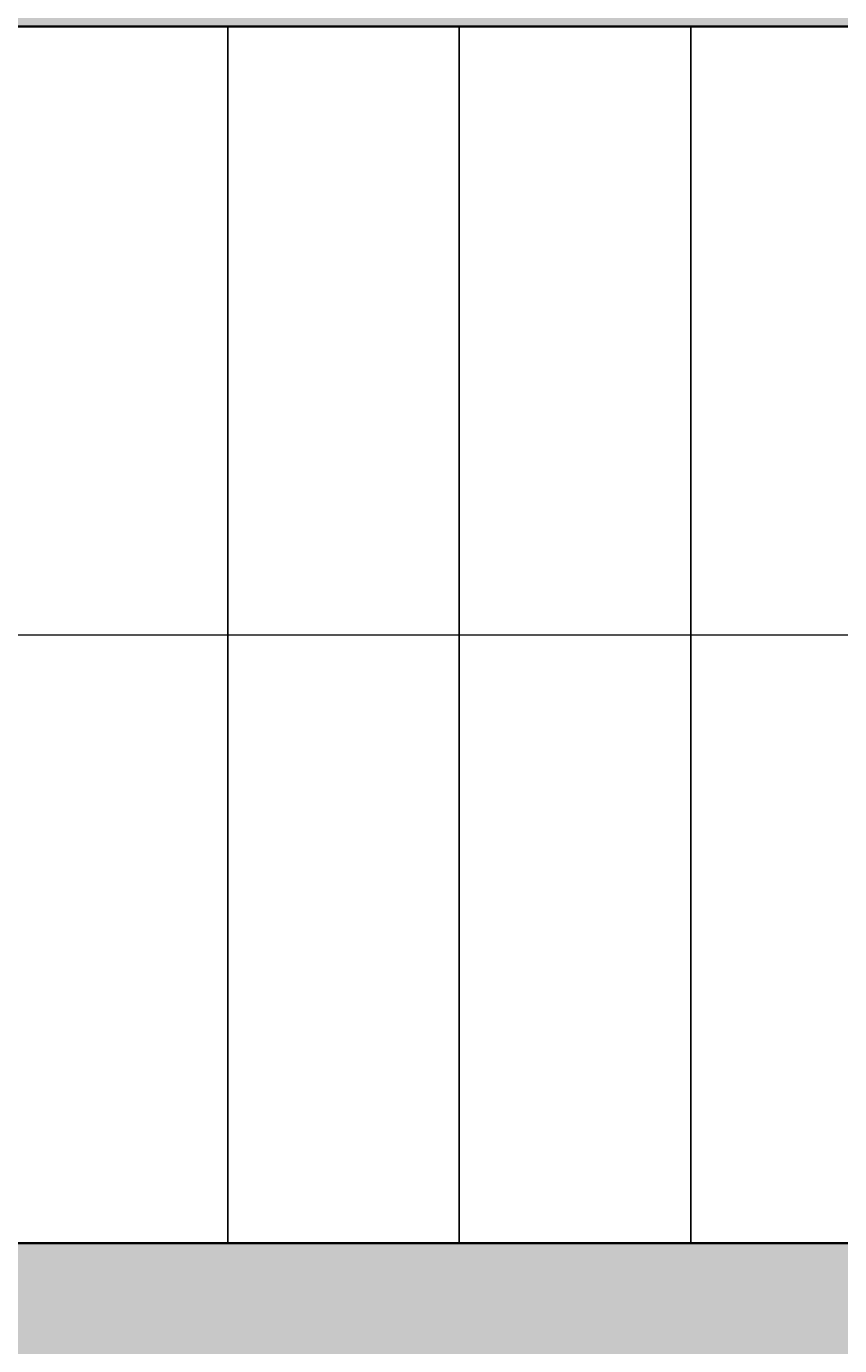
# Model space of a CAD drawing. Units: inches. Extents: x 1998 to 2588, y 1139 to 1977.
# Tile 89 of 134: x 2425 to 2453, y 1477 to 1523. Entities that reach past the tile are written whole.
import ezdxf

# ---------------------------------------------------------------- set-up
doc = ezdxf.new("R2010")
doc.units = ezdxf.units.IN
for name, color, linetype, lineweight in [('A-ANNO-DIMS', 2, 'Continuous', 18), ('A-ANNO-SYMB', 7, 'Continuous', 18), ('A-FLOR-EVTR', 7, 'Continuous', 35), ('A-FLOR-STRS', 7, 'Continuous', 25), ('A-WALL-PATT', 252, 'Continuous', 13), ('WALL', 200, 'Continuous', 35)]:
    doc.layers.add(name, color=color, linetype=linetype, lineweight=lineweight)
doc.styles.get("Standard").update_dxf_attribs({"font": 'arial.ttf'})
doc.dimstyles.get("Standard").update_dxf_attribs({"dimtxt": 0.18, "dimasz": 0.18, "dimexe": 0.18, "dimexo": 0.0625, "dimgap": 0.09, "dimtad": 0, "dimtih": 1, "dimtoh": 1, "dimdec": 4, "dimzin": 0, "dimdsep": 46, "dimtxsty": 'Standard', "dimcen": 0.09, "dimadec": 0, "dimazin": 0, "dimtfac": 1, "dimtdec": 4, "dimtofl": 0, "dimtmove": 0, "dimatfit": 3, "dimfxl": 1, "dimtolj": 1, "dimtzin": 0, "dimarcsym": 0})

# ---------------------------------------------------------------- blocks, each defined once
blk = doc.blocks.new('*D24')
at = {"layer": 'A-ANNO-DIMS', "color": 0, "lineweight": -2, "transparency": 16777216}
for p, q in [((2398.535, 1911.232), (2588.309, 1911.232)), ((2588.129, 1911.052), (2588.129, 1570.164)), ((2588.129, 1228.912), (2588.129, 1569.8)), ((2527.535, 1228.732), (2588.309, 1228.732))]:
    blk.add_line(p, q, dxfattribs=at)
at = {"layer": 'A-ANNO-DIMS', "color": 0, "transparency": 16777216}
for points in [[(2588.099, 1911.052), (2588.159, 1911.052), (2588.129, 1911.232)], [(2588.099, 1228.912), (2588.159, 1228.912), (2588.129, 1228.732)]]:
    blk.add_solid(points, dxfattribs=at)
at = {"layer": 'Defpoints', "color": 0, "transparency": 16777216}
for p in [(2398.473, 1911.232), (2588.129, 1911.232), (2527.473, 1228.732)]:
    blk.add_point(p, dxfattribs=at)
at = {"layer": 'A-ANNO-DIMS', "color": 0, "transparency": 16777216, "insert": (2588.129, 1569.982), "char_height": 0.18, "attachment_point": 5}
blk.add_mtext('\\A1;682.5', dxfattribs=at)
blk = doc.blocks.new('*D33')
at = {"layer": 'A-ANNO-DIMS', "color": 0, "lineweight": -2, "transparency": 16777216}
for p, q in [((2407.973, 1480.67), (2407.973, 1138.602)), ((2498.179, 1480.67), (2498.179, 1138.602)), ((2408.153, 1138.782), (2452.753, 1138.782)), ((2497.999, 1138.782), (2453.399, 1138.782))]:
    blk.add_line(p, q, dxfattribs=at)
at = {"layer": 'A-ANNO-DIMS', "color": 0, "transparency": 16777216}
for points in [[(2408.153, 1138.812), (2408.153, 1138.752), (2407.973, 1138.782)], [(2497.999, 1138.812), (2497.999, 1138.752), (2498.179, 1138.782)]]:
    blk.add_solid(points, dxfattribs=at)
at = {"layer": 'Defpoints', "color": 0, "transparency": 16777216}
for p in [(2407.973, 1480.732), (2498.179, 1480.732), (2498.179, 1138.782)]:
    blk.add_point(p, dxfattribs=at)
at = {"layer": 'A-ANNO-DIMS', "color": 0, "transparency": 16777216, "insert": (2453.076, 1138.782), "char_height": 0.18, "attachment_point": 5}
blk.add_mtext('\\A1;90.2', dxfattribs=at)

msp = doc.modelspace()

# ---------------------------------------------------------------- hatches: boundary and pattern name
at = {"layer": 'A-WALL-PATT'}
h = msp.add_hatch(color=256, dxfattribs=at)
h.dxf.hatch_style = 1
h.paths.add_polyline_path([(2527.4729, 1362.2324), (2510.9729, 1362.2324), (2510.9729, 1357.7324), (2518.4729, 1357.7324), (2518.4729, 1237.7324), (2503.1458, 1237.7324), (2503.1458, 1228.7324), (2527.4729, 1228.7324)])
h.paths.add_polyline_path([(2490.5682, 1362.2324), (2398.4729, 1362.2324), (2398.4729, 1357.7324), (2490.5682, 1357.7324)])
h.paths.add_polyline_path([(2224.9729, 1264.7324), (2222.9729, 1264.7324), (2222.9729, 1232.4125), (2341.4729, 1232.4125), (2341.4729, 1234.4125), (2224.9729, 1234.4125)])
h.paths.add_polyline_path([(2334.5332, 1273.7324), (2264.7638, 1273.7324), (2264.7638, 1269.5611, -0.043659), (2264.3413, 1264.7324), (2334.5332, 1264.7324)])
h.paths.add_polyline_path([(2236.9551, 1273.7324), (2234.4125, 1273.7324), (2234.4125, 1264.7324), (2236.9551, 1264.7324), (2236.9551, 1269.5611)])
h.paths.add_polyline_path([(2222.9729, 1293.2324), (2096.9729, 1293.2324), (2096.9729, 1345.0966), (2087.9729, 1345.0966), (2087.9729, 1284.2324), (2222.9729, 1284.2324), (2222.9729, 1285.137)])
h.paths.add_polyline_path([(2096.9729, 1458.7927), (2087.9729, 1458.7927), (2087.9729, 1417.7324), (2087.9729, 1413.2324), (2096.9729, 1413.2324), (2096.9729, 1417.7324)])
h.paths.add_polyline_path([(2096.9729, 1413.2324), (2087.9729, 1413.2324), (2087.9729, 1365.5012), (2096.9729, 1365.5012), (2096.9729, 1369.3358)])
h.paths.add_polyline_path([(2186.2943, 1417.7324), (2138.6074, 1417.7324), (2096.9729, 1417.7324), (2096.9729, 1413.2324), (2138.6074, 1413.2324), (2186.2943, 1413.2324)])
h.paths.add_polyline_path([(2181.4729, 1465.7324), (2176.9729, 1465.7324), (2176.9729, 1451.6434), (2181.4729, 1451.6434)])
h.paths.add_polyline_path([(2181.4729, 1422.1664), (2176.9729, 1422.1664), (2176.9729, 1417.7324), (2181.4729, 1417.7324)])
h.paths.add_polyline_path([(2063.9729, 1465.7324), (2087.9729, 1465.7324), (2087.9729, 1470.2324), (2059.4729, 1470.2324), (2059.4729, 1413.2324), (2087.9729, 1413.2324), (2087.9729, 1417.7324), (2063.9729, 1417.7324)])
h.paths.add_polyline_path([(2181.4729, 1755.2324), (2176.9729, 1755.2324), (2176.9729, 1748.6798), (2177.0513, 1748.6798), (2181.4729, 1748.6798)])
h.paths.add_polyline_path([(2227.4729, 1707.2324), (2220.4647, 1707.2324), (2220.4647, 1702.7324), (2222.9729, 1702.7324), (2222.9729, 1604.637), (2227.4729, 1604.637)])
h.paths.add_polyline_path([(2114.9729, 1702.7324), (2105.9729, 1702.7324), (2105.9729, 1628.4781, -0.0318759), (2110.1012, 1628.7416), (2114.9729, 1628.7416)])
h.paths.add_polyline_path([(2345.9729, 1739.3278), (2341.4729, 1739.3278), (2341.4729, 1647.5211), (2345.9729, 1647.5211)])
h.paths.add_polyline_path([(2350.6273, 1641.2324), (2345.9729, 1641.2324), (2345.9729, 1636.7324), (2350.6273, 1636.7324), (2350.6273, 1639.8729)])
h.paths.add_polyline_path([(2501.9729, 1641.2324), (2407.9729, 1641.2324), (2392.5005, 1641.2324), (2392.5005, 1639.8729), (2392.5005, 1636.7324), (2501.9729, 1636.7324)])
h.paths.add_polyline_path([(2510.9729, 1755.2324), (2501.9729, 1755.2324), (2501.9729, 1641.2324), (2510.9729, 1641.2324)])
h.paths.add_polyline_path([(2549.1786, 1641.2324), (2522.3775, 1641.2324), (2522.3775, 1636.7324), (2540.1786, 1636.7324), (2540.1786, 1480.7324), (2522.3775, 1480.7324), (2522.3775, 1476.2324), (2549.1786, 1476.2324)])
h.paths.add_polyline_path([(2498.1786, 1594.7324), (2407.9729, 1594.7324), (2407.9729, 1585.7324), (2416.9729, 1585.7324), (2489.1786, 1585.7324), (2489.1786, 1531.7324), (2416.9729, 1531.7324), (2407.9729, 1531.7324), (2407.9729, 1522.7324), (2498.1786, 1522.7324)])
h.paths.add_polyline_path([(2351.6437, 1480.7324), (2345.9729, 1480.7324), (2345.9729, 1476.2324), (2351.6437, 1476.2324), (2351.6437, 1477.5919)])
h.paths.add_polyline_path([(2501.9729, 1480.7324), (2498.1786, 1480.7324), (2407.9729, 1480.7324), (2393.5168, 1480.7324), (2393.5168, 1477.5919), (2393.5168, 1476.2324), (2501.9729, 1476.2324)])

# ---------------------------------------------------------------- linework, layer by layer
at = {"layer": 'A-ANNO-SYMB'}
msp.add_line((2407.9729, 1501.7324), (2498.1786, 1501.7324), dxfattribs=at)
at = {"layer": 'A-FLOR-EVTR'}
msp.add_lwpolyline([(2407.9729, 1522.7324), (2498.1786, 1522.7324), (2498.1786, 1594.7324), (2407.9729, 1594.7324)], close=True, dxfattribs=at)
at = {"layer": 'A-FLOR-STRS'}
for p, q in [((2540.1786, 1522.7324), (2407.9729, 1522.7324)), ((2431.9729, 1480.7324), (2431.9729, 1522.7324)), ((2439.9729, 1480.7324), (2439.9729, 1522.7324)), ((2447.9729, 1480.7324), (2447.9729, 1522.7324))]:
    msp.add_line(p, q, dxfattribs=at)
at = {"layer": 'WALL'}
msp.add_line((2540.1786, 1480.7324), (2407.9729, 1480.7324), dxfattribs=at)

# ---------------------------------------------------------------- dimensions: what is measured, and where the dimension line sits
at = {"layer": 'A-ANNO-DIMS'}
dim = msp.add_linear_dim(base=(2588.1286, 1911.2324), p1=(2527.4729, 1228.7324), p2=(2398.4729, 1911.2324), angle=90, dimstyle='Standard', override={"dimdec": 1, "dimlfac": 1, "dimrnd": 0, "dimzin": 0, "dimdsep": 46, "dimlunit": 2}, dxfattribs=at)
dim.commit()
dim.dimension.update_dxf_attribs({"geometry": '*D24', "text_midpoint": (2588.1286, 1569.9824)})
dim = msp.add_linear_dim(base=(2498.1786, 1138.7824), p1=(2407.9729, 1480.7324), p2=(2498.1786, 1480.7324), dimstyle='Standard', override={"dimdec": 1, "dimlfac": 1, "dimrnd": 0, "dimzin": 0, "dimdsep": 46, "dimlunit": 2}, dxfattribs=at)
dim.commit()
dim.dimension.update_dxf_attribs({"geometry": '*D33', "text_midpoint": (2453.0757, 1138.7824)})

doc.saveas('drawing.dxf')
